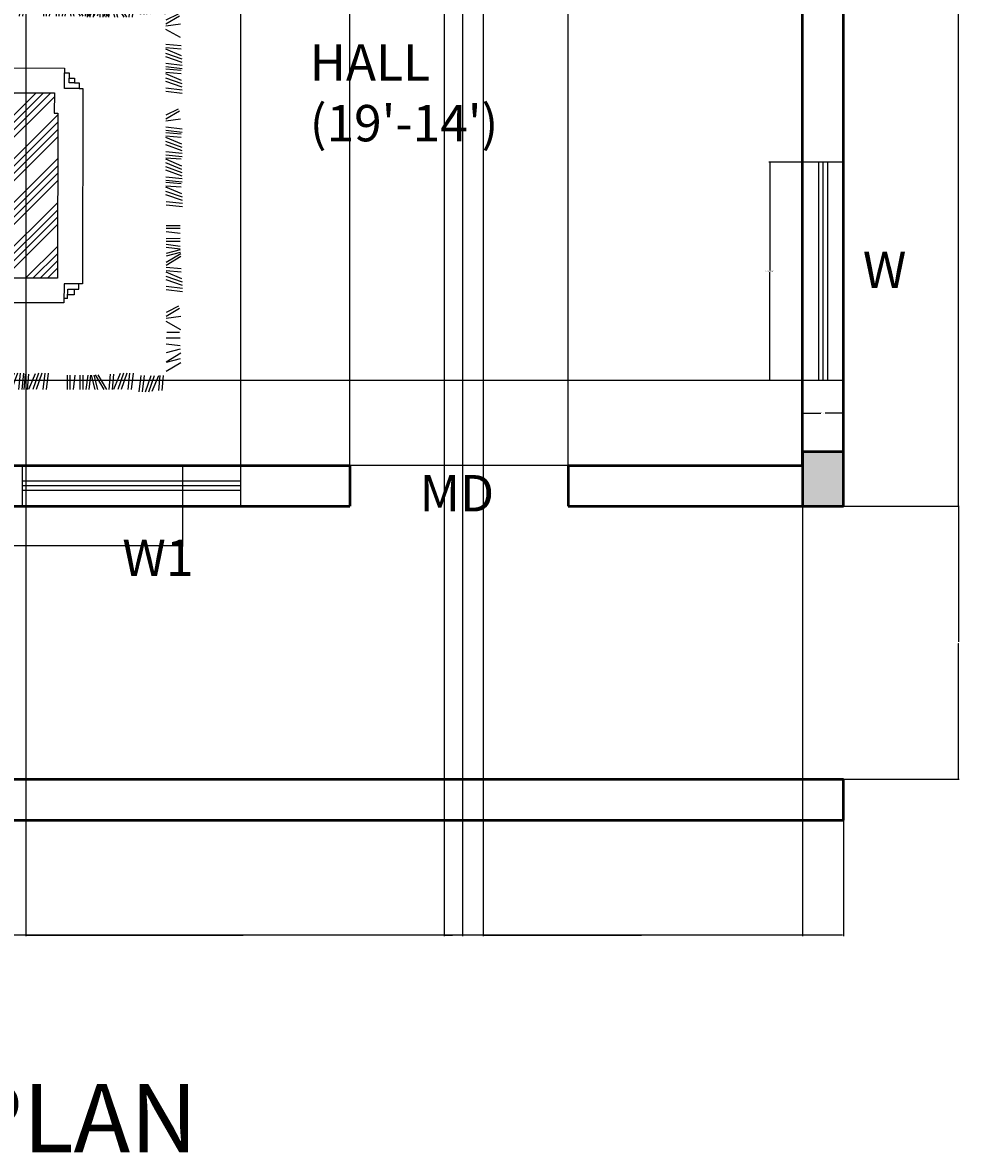
# Model space of a CAD drawing. Units: inches. Extents: x -1517 to -668, y -425 to 52.
# Tile 6 of 13: x -1186 to -980, y -425 to -176. Entities that reach past the tile are written whole.
import ezdxf

# ---------------------------------------------------------------- set-up
doc = ezdxf.new("R2010")
doc.units = ezdxf.units.IN
doc.header["$MEASUREMENT"] = 0
for name, color, linetype, lineweight in [('A-ANNO-DIMS', 2, 'Continuous', 18), ('A-ANNO-TEXT', 7, 'Continuous', 18), ('A-AREA-IDEN', 7, 'Continuous', 25), ('A-COLS-PATT', 252, 'Continuous', 13), ('column', 7, 'Continuous', 50), ('furniture block', 8, 'Continuous', 18), ('walls', 240, 'Continuous', 50), ('windows', 140, 'Continuous', 25)]:
    doc.layers.add(name, color=color, linetype=linetype, lineweight=lineweight)
for name, color, linetype in [('复线', 6, 'Continuous'), ('家具', 4, 'Continuous'), ('辅助线', 1, 'Continuous'), ('门窗', 2, 'Continuous')]:
    doc.layers.add(name, color=color, linetype=linetype)
doc.styles.get("Standard").update_dxf_attribs({"font": 'arial.ttf'})
doc.dimstyles.get("Standard").update_dxf_attribs({"dimtxt": 0.18, "dimasz": 0.18, "dimexe": 0.18, "dimexo": 0.0625, "dimgap": 0.09, "dimtad": 0, "dimtih": 1, "dimtoh": 1, "dimdec": 4, "dimzin": 0, "dimdsep": 46, "dimlunit": 4, "dimtxsty": 'Standard', "dimcen": 0.09, "dimadec": 0, "dimazin": 0, "dimtfac": 1, "dimtdec": 4, "dimtofl": 0, "dimtmove": 0, "dimatfit": 3, "dimfxl": 1, "dimtolj": 1, "dimtzin": 0, "dimarcsym": 0})

# ---------------------------------------------------------------- blocks, each defined once
blk = doc.blocks.new('column')
for p, q in [((0, 9), (0, 0)), ((12, 9), (0, 9)), ((12, 0), (12, 9)), ((0, 0), (12, 0))]:
    blk.add_line(p, q)
blk = doc.blocks.new('window 4ft')
for p, q in [((0, 9), (0, 0)), ((48, 9), (48, 0)), ((0, 5.5), (48, 5.5)), ((0, 4.5), (48, 4.5)), ((0, 3.5), (48, 3.5))]:
    blk.add_line(p, q)
blk = doc.blocks.new('A$C2A9E403C')
at = {"layer": '复线'}
for p, q in [((-0.6124, 1.2901), (-0.6119, 1.5387)), ((-0.6119, 1.5387), (-0.4956, 1.5385)), ((-0.4956, 1.5596), (0.4554, 1.5575)), ((-0.4956, 1.5385), (-0.4956, 1.5596)), ((0.4554, 1.5575), (0.4547, 1.198)), ((-0.5913, 1.2901), (-0.6124, 1.2901)), ((-0.5915, 1.1738), (-0.5913, 1.2901)), ((0.3437, 1.1718), (-0.5915, 1.1738)), ((0.3437, 1.1982), (0.3437, 1.1718)), ((0.4547, 1.198), (0.3437, 1.1982)), ((0.7969, 0.7406), (-0.7994, 0.7387)), ((-0.27, 0.7177), (-0.7787, 0.7173)), ((-0.7787, 0.7173), (-0.7783, 0.1924)), ((-0.2696, 0.1928), (-0.27, 0.7177)), ((0.2616, 0.7183), (-0.2471, 0.718)), ((-0.2471, 0.718), (-0.2468, 0.1931)), ((0.2619, 0.1934), (0.2616, 0.7183)), ((0.7846, 0.7189), (0.2759, 0.7186)), ((0.2759, 0.7186), (0.2762, 0.1937)), ((0.785, 0.194), (0.7846, 0.7189)), ((-1.3039, 0.62), (-1.3039, 0.3666)), ((1.2704, 0.6186), (1.2704, 0.3652)), ((-1.1772, 0.4933), (-1.4306, 0.4933)), ((1.3971, 0.4919), (1.1437, 0.4919)), ((-0.7783, 0.1924), (-0.2696, 0.1928)), ((-0.2468, 0.1931), (0.2619, 0.1934)), ((0.2762, 0.1937), (0.785, 0.194))]:
    blk.add_line(p, q, dxfattribs=at)
for centre in [(-1.2867, 0.4933), (1.2877, 0.4919)]:
    blk.add_circle(centre, 0.0634, dxfattribs=at)
at = {"layer": '家具'}
for p, q in [((0.6497, 2.19), (0.6526, 2.1827)), ((-0.6379, 1.6813), (-0.6378, 1.7025)), ((-0.6378, 1.7025), (0.4874, 1.7)), ((0.4874, 1.7), (0.4872, 1.5943)), ((-0.6961, 1.655), (-0.6696, 1.655)), ((-0.6961, 1.6233), (-0.6961, 1.655)), ((-0.6696, 1.6814), (-0.6379, 1.6813)), ((-0.6696, 1.655), (-0.6696, 1.6814)), ((-0.6694, 1.655), (-0.6694, 1.6235)), ((-0.6378, 1.6814), (-0.6379, 1.597)), ((0.519, 1.6788), (0.4873, 1.6789)), ((0.5189, 1.6154), (0.519, 1.6788)), ((0.519, 1.6524), (0.5507, 1.6523)), ((0.5507, 1.6523), (0.5506, 1.6153)), ((-0.7553, 1.1479), (-0.7543, 1.597)), ((-0.7543, 1.597), (-0.7279, 1.597)), ((-0.6379, 1.597), (-0.7282, 1.5972)), ((-0.7279, 1.597), (-0.7278, 1.6234)), ((-0.7278, 1.6234), (-0.6961, 1.6233)), ((-0.6694, 1.6235), (-0.6966, 1.6235)), ((0.4872, 1.5943), (0.5981, 1.5941)), ((0.5717, 1.6153), (0.5189, 1.6154)), ((0.5717, 1.6153), (0.5717, 1.5941)), ((0.5981, 1.5941), (0.5971, 1.1396)), ((-0.7341, 1.1478), (-0.7553, 1.1479)), ((-0.6393, 1.1482), (-0.7352, 1.1484)), ((-0.7342, 1.1161), (-0.7341, 1.1478)), ((-0.7342, 1.1161), (-0.6972, 1.116)), ((-0.6709, 1.116), (-0.6979, 1.1161)), ((-0.6973, 1.0896), (-0.6972, 1.116)), ((-0.6709, 1.0896), (-0.6709, 1.116)), ((-0.6394, 1.058), (-0.6393, 1.1482)), ((0.4862, 1.1399), (0.4859, 1.0289)), ((0.4862, 1.1399), (0.5971, 1.1396)), ((0.5177, 1.0553), (0.5178, 1.1134)), ((0.5178, 1.1134), (0.5706, 1.1133)), ((0.5442, 1.1133), (0.5441, 1.0816)), ((0.5707, 1.1397), (0.5706, 1.1133)), ((-0.6709, 1.0896), (-0.6973, 1.0896)), ((-0.671, 1.0579), (-0.6709, 1.0896)), ((-0.6393, 1.0578), (-0.671, 1.0579)), ((-0.6393, 1.0314), (-0.6393, 1.0578)), ((0.5177, 1.0553), (0.486, 1.0553)), ((0.5441, 1.0816), (0.5177, 1.0817)), ((0.4859, 1.0289), (-0.6393, 1.0314)), ((-1.549, 0.751), (-1.0422, 0.7516)), ((-1.5485, 0.2441), (-1.549, 0.751)), ((-1.0422, 0.7516), (-1.0416, 0.2447)), ((-0.9818, 0.2137), (-0.9824, 0.7352)), ((-0.7945, 0.7328), (-0.7941, 0.1426)), ((0.7969, 0.7406), (0.7973, 0.1532)), ((0.9782, 0.2083), (0.9775, 0.741)), ((1.0263, 0.7379), (1.5332, 0.7385)), ((1.0269, 0.2311), (1.0263, 0.7379)), ((1.5332, 0.7385), (1.5338, 0.2316)), ((-1.0416, 0.2447), (-1.5485, 0.2441)), ((1.5338, 0.2316), (1.0269, 0.2311)), ((-0.7773, -0.0005), (0.7773, 0.0005))]:
    blk.add_line(p, q, dxfattribs=at)
for centre in [(-1.3039, 0.4933), (1.2704, 0.4919)]:
    blk.add_circle(centre, 0.1267, dxfattribs=at)
for centre, radius, start, end in [((-0.8894, 0.6597), 0.1198, 37.63003, 140.94625), ((0.8885, 0.6609), 0.1198, 41.79306, 142.44625), ((-0.7672, 0.2138), 0.2146, 180.03814, 267.3174), ((0.7771, 0.2016), 0.2011, 270.03814, 1.88757), ((-0.6554, -0.0689), 0.253, 103.34083, 123.25708), ((-0.3975, -0.0687), 0.253, 56.82018, 76.73545), ((-0.1227, -0.0686), 0.253, 59.39874, 122.94271), ((0.1299, -0.0495), 0.2341, 53.21137, 121.92426), ((0.4167, -0.0682), 0.253, 103.34083, 125.41455), ((0.6746, -0.068), 0.253, 60.98187, 76.73545)]:
    blk.add_arc(centre, radius, start, end, dxfattribs=at)
at = {"layer": '辅助线'}
for p, q in [((-1.0661, 2.2523), (-1.0302, 2.1808)), ((-1.0533, 2.2588), (-1.0079, 2.1808)), ((-1.0082, 2.2653), (-0.9957, 2.1808)), ((-0.9309, 2.2654), (-0.9778, 2.1808)), ((-0.8827, 2.2686), (-0.8899, 2.1809)), ((-0.8633, 2.2687), (-0.8705, 2.181)), ((-0.8247, 2.2719), (-0.8633, 2.181)), ((-0.8054, 2.2752), (-0.8391, 2.181)), ((-0.7861, 2.2752), (-0.8197, 2.181)), ((-0.77, 2.2752), (-0.7803, 2.1811)), ((-0.7507, 2.2752), (-0.761, 2.1811)), ((-0.741, 2.2688), (-0.7482, 2.1811)), ((-0.7217, 2.2688), (-0.7289, 2.1811)), ((-0.6831, 2.2721), (-0.7216, 2.1811)), ((-0.6638, 2.2753), (-0.6974, 2.1812)), ((-0.6444, 2.2753), (-0.6781, 2.1812)), ((-0.6284, 2.2754), (-0.6387, 2.1812)), ((-0.609, 2.2754), (-0.6194, 2.1812)), ((-0.5189, 2.253), (-0.483, 2.1814)), ((-0.506, 2.2594), (-0.4607, 2.1814)), ((-0.4609, 2.2659), (-0.4484, 2.1814)), ((-0.4036, 2.2756), (-0.414, 2.1815)), ((-0.3843, 2.2757), (-0.3946, 2.1815)), ((-0.3746, 2.2692), (-0.3818, 2.1815)), ((-0.3553, 2.2693), (-0.3625, 2.1815)), ((-0.3167, 2.2725), (-0.3552, 2.1816)), ((-0.2974, 2.2758), (-0.331, 2.1816)), ((-0.278, 2.2758), (-0.3117, 2.1816)), ((-0.262, 2.2758), (-0.2723, 2.1816)), ((-0.2426, 2.2758), (-0.253, 2.1817)), ((-0.2292, 2.2694), (-0.2364, 2.1817)), ((-0.1906, 2.2727), (-0.2291, 2.1817)), ((-0.1712, 2.2727), (-0.2098, 2.1817)), ((-0.1519, 2.2759), (-0.1856, 2.1817)), ((-0.1326, 2.2759), (-0.1663, 2.1818)), ((-0.1165, 2.276), (-0.1269, 2.1818)), ((-0.0972, 2.276), (-0.1076, 2.1818)), ((-0.0875, 2.2696), (-0.0948, 2.1819)), ((-0.0682, 2.2696), (-0.0754, 2.1819)), ((-0.0296, 2.2728), (-0.0682, 2.1819)), ((-0.0103, 2.2761), (-0.044, 2.1819)), ((0.009, 2.2761), (-0.0246, 2.1819)), ((0.0251, 2.2761), (0.0148, 2.182)), ((0.0444, 2.2761), (0.0341, 2.182)), ((0.1539, 2.2634), (0.154, 2.1821)), ((0.17, 2.2634), (0.1701, 2.1822)), ((0.199, 2.2635), (0.1882, 2.1822)), ((0.2279, 2.2635), (0.228, 2.1822)), ((0.244, 2.2635), (0.2441, 2.1822)), ((0.273, 2.2635), (0.2623, 2.1823)), ((0.2891, 2.2636), (0.2783, 2.1823)), ((0.2923, 2.2636), (0.3127, 2.1823)), ((0.3084, 2.2636), (0.3288, 2.1823)), ((0.3148, 2.2668), (0.3657, 2.1824)), ((0.3309, 2.2668), (0.3818, 2.1824)), ((0.4018, 2.2701), (0.3945, 2.1824)), ((0.4211, 2.2702), (0.4139, 2.1824)), ((0.4597, 2.2734), (0.4211, 2.1825)), ((0.479, 2.2767), (0.4453, 2.1825)), ((0.4983, 2.2767), (0.4647, 2.1825)), ((0.5144, 2.2767), (0.5041, 2.1825)), ((0.5337, 2.2767), (0.5234, 2.1826)), ((0.6175, 2.2543), (0.6497, 2.19)), ((0.6303, 2.2607), (0.6756, 2.1827)), ((0.6754, 2.2672), (0.6879, 2.1828)), ((0.7526, 2.2673), (0.7058, 2.1828)), ((0.7668, 2.187), (0.7667, 2.2602)), ((0.8009, 2.2642), (0.801, 2.1829)), ((0.846, 2.2642), (0.8352, 2.1829)), ((0.8653, 2.2642), (0.8857, 2.183)), ((0.8878, 2.2675), (0.9387, 2.1831)), ((0.92, 2.2643), (0.9405, 2.1831)), ((0.9426, 2.2675), (0.9934, 2.1831)), ((-1.1526, 2.1822), (-1.0649, 2.175)), ((1.1031, 2.1597), (1.0154, 2.1669)), ((-1.1494, 2.1339), (-1.0648, 2.0871)), ((1.1031, 2.1404), (1.0154, 2.1476)), ((1.1064, 2.1018), (1.0154, 2.1404)), ((1.1096, 2.0825), (1.0155, 2.1161)), ((1.1097, 2.0632), (1.0155, 2.0968)), ((-1.1493, 2.0567), (-1.0648, 2.0692)), ((-1.1428, 2.0116), (-1.0648, 2.0569)), ((-1.1205, 2.0067), (-1.0648, 2.0347)), ((1.1097, 2.0471), (1.0155, 2.0574)), ((1.1097, 2.0278), (1.0156, 2.0381)), ((-1.1354, 1.9942), (-1.0477, 1.987)), ((-1.1354, 1.9749), (-1.0477, 1.9677)), ((-1.1321, 1.9041), (-1.0476, 1.9549)), ((1.0017, 1.9919), (1.0958, 1.9816)), ((1.0017, 1.9726), (1.0958, 1.9623)), ((1.0017, 1.9565), (1.0959, 1.9229)), ((-1.132, 1.888), (-1.0476, 1.9389)), ((-1.1288, 1.8816), (-1.0476, 1.902)), ((1.0017, 1.9372), (1.0959, 1.9036)), ((1.005, 1.9179), (1.0959, 1.8793)), ((-1.1487, 1.855), (-1.0545, 1.8446)), ((-1.1486, 1.8356), (-1.0545, 1.8253)), ((-1.1288, 1.8655), (-1.0476, 1.8859)), ((-1.1288, 1.8623), (-1.0475, 1.8515)), ((-1.1288, 1.8462), (-1.0475, 1.8354)), ((1.0082, 1.8793), (1.0959, 1.8721)), ((1.0083, 1.86), (1.096, 1.8528)), ((1.0116, 1.7892), (1.096, 1.84)), ((1.0116, 1.7731), (1.096, 1.8239)), ((-1.1486, 1.8196), (-1.0544, 1.7859)), ((-1.1486, 1.8002), (-1.0544, 1.7666)), ((-1.1454, 1.7809), (-1.0544, 1.7424)), ((-1.1287, 1.8172), (-1.0475, 1.8173)), ((-1.1287, 1.8011), (-1.0475, 1.8012)), ((-1.1287, 1.7721), (-1.0474, 1.7614)), ((1.0148, 1.7666), (1.096, 1.787)), ((1.0148, 1.7505), (1.0961, 1.771)), ((-1.1421, 1.7423), (-1.0544, 1.7351)), ((-1.1421, 1.723), (-1.0544, 1.7158)), ((-1.1388, 1.6522), (-1.0544, 1.703)), ((-1.1287, 1.7432), (-1.0474, 1.7433)), ((-1.1286, 1.7271), (-1.0474, 1.7272)), ((1.0148, 1.7473), (1.0961, 1.7366)), ((1.0148, 1.7312), (1.0961, 1.7205)), ((1.0149, 1.7022), (1.0961, 1.7023)), ((-1.1388, 1.6361), (-1.0543, 1.6869)), ((-1.1355, 1.6296), (-1.0543, 1.6501)), ((-1.1355, 1.6135), (-1.0543, 1.634)), ((1.0149, 1.6861), (1.0962, 1.6862)), ((1.0149, 1.6572), (1.0962, 1.6464)), ((1.015, 1.6282), (1.0962, 1.6283)), ((-1.1355, 1.6103), (-1.0542, 1.5996)), ((-1.1355, 1.5942), (-1.0542, 1.5835)), ((-1.1355, 1.5653), (-1.0542, 1.5654)), ((1.015, 1.6121), (1.0962, 1.6122)), ((-1.1354, 1.5492), (-1.0542, 1.5493)), ((-1.1354, 1.5202), (-1.0541, 1.5094)), ((-0.2678, 1.1731), (-0.6119, 1.5187)), ((-0.2258, 1.173), (-0.5898, 1.5387)), ((-0.0998, 1.1727), (-0.4849, 1.5596)), ((-0.0578, 1.1727), (-0.4429, 1.5595)), ((-0.0158, 1.1726), (-0.4009, 1.5594)), ((0.0262, 1.1725), (-0.3589, 1.5593)), ((0.1522, 1.1722), (-0.2329, 1.559)), ((0.1942, 1.1721), (-0.1909, 1.5589)), ((0.2362, 1.172), (-0.1489, 1.5588)), ((0.2782, 1.1719), (-0.1069, 1.5587)), ((0.3779, 1.1981), (0.0191, 1.5585)), ((0.4199, 1.198), (0.0611, 1.5584)), ((0.4547, 1.2052), (0.1031, 1.5583)), ((0.4548, 1.2472), (0.1451, 1.5582)), ((0.455, 1.3732), (0.2711, 1.5579)), ((0.4551, 1.4152), (0.3131, 1.5578)), ((0.4552, 1.4572), (0.3551, 1.5577)), ((0.4553, 1.4992), (0.3971, 1.5576)), ((1.0022, 1.5026), (1.0964, 1.4923)), ((-1.1354, 1.4912), (-1.0541, 1.4913)), ((-1.1354, 1.4751), (-1.0541, 1.4752)), ((-0.3518, 1.1733), (-0.6121, 1.4347)), ((-0.3098, 1.1732), (-0.612, 1.4767)), ((1.0023, 1.4833), (1.0964, 1.473)), ((1.0023, 1.4672), (1.0965, 1.4336)), ((1.0023, 1.4479), (1.0965, 1.4143)), ((1.0055, 1.4286), (1.0965, 1.39)), ((1.0088, 1.39), (1.0965, 1.3828)), ((1.0088, 1.3707), (1.0965, 1.3635)), ((-1.1481, 1.3657), (-1.0539, 1.3553)), ((-1.1481, 1.3463), (-1.0539, 1.336)), ((-1.1481, 1.3303), (-1.0539, 1.2966)), ((-1.148, 1.3109), (-1.0539, 1.2773)), ((-0.5938, 1.2901), (-0.6124, 1.3087)), ((1.0024, 1.361), (1.0966, 1.3506)), ((1.0024, 1.3417), (1.0966, 1.3313)), ((1.0024, 1.3256), (1.0966, 1.2919)), ((1.0025, 1.3063), (1.0966, 1.2726)), ((-1.1448, 1.2916), (-1.0538, 1.2531)), ((-1.1415, 1.253), (-1.0538, 1.2458)), ((-0.5198, 1.1737), (-0.5914, 1.2456)), ((-0.4778, 1.1736), (-0.5913, 1.2876)), ((1.0057, 1.287), (1.0967, 1.2484)), ((1.0057, 1.2677), (1.0967, 1.2291)), ((-1.1479, 1.224), (-1.0538, 1.2137)), ((-1.1479, 1.2047), (-1.0538, 1.1944)), ((-1.1479, 1.1886), (-1.0537, 1.155)), ((-1.1415, 1.2337), (-1.0538, 1.2265)), ((-0.5618, 1.1738), (-0.5915, 1.2036)), ((1.0026, 1.2156), (1.0967, 1.2052)), ((1.0026, 1.1963), (1.0967, 1.1859)), ((1.0026, 1.1802), (1.0968, 1.1465)), ((1.009, 1.229), (1.0967, 1.2218)), ((-1.1479, 1.1693), (-1.0537, 1.1356)), ((-1.1446, 1.15), (-1.0537, 1.1114)), ((-1.1446, 1.1307), (-1.0536, 1.0921)), ((1.0026, 1.1608), (1.0968, 1.1272)), ((1.0059, 1.1415), (1.0968, 1.103)), ((-1.1478, 1.0786), (-1.0536, 1.0682)), ((-1.1477, 1.0593), (-1.0536, 1.0489)), ((-1.1477, 1.0432), (-1.0535, 1.0095)), ((-1.1413, 1.0921), (-1.0536, 1.0848)), ((1.0027, 1.0739), (1.0969, 1.0636)), ((1.0028, 1.0546), (1.0969, 1.0443)), ((1.0091, 1.1029), (1.0968, 1.0957)), ((1.0092, 1.0836), (1.0969, 1.0764)), ((-1.1477, 1.0239), (-1.0535, 0.9902)), ((-1.1445, 1.0046), (-1.0535, 0.966)), ((1.0125, 0.9973), (1.0969, 1.0098)), ((1.019, 0.9522), (1.097, 0.9975)), ((-1.1476, 0.937), (-1.0535, 0.9266)), ((-1.1476, 0.9176), (-1.0534, 0.9073)), ((-1.1412, 0.9659), (-1.0535, 0.9587)), ((-1.1412, 0.9466), (-1.0535, 0.9394)), ((1.0182, 0.9266), (1.1091, 0.8881)), ((1.0254, 0.9393), (1.097, 0.9752)), ((-1.1379, 0.8603), (-1.0534, 0.8728)), ((-1.1314, 0.8152), (-1.0534, 0.8605)), ((1.015, 0.8745), (1.1091, 0.8642)), ((1.015, 0.8552), (1.1092, 0.8449)), ((1.0214, 0.888), (1.1091, 0.8808)), ((-1.1353, 0.8078), (-1.062, 0.8079)), ((-1.132, 0.8163), (-1.0631, 0.7916)), ((-1.1249, 0.8024), (-1.0533, 0.8383)), ((-1.0607, 0.8176), (-1.0606, 0.7516)), ((1.015, 0.8391), (1.1092, 0.8055)), ((1.0151, 0.7984), (1.0863, 0.8153)), ((1.0173, 0.7141), (1.0171, 0.8166)), ((1.0174, 0.7888), (1.0906, 0.7889)), ((-1.5237, 0.7257), (-1.0675, 0.7262)), ((-1.5231, 0.2695), (-1.5237, 0.7257)), ((-1.1351, 0.7732), (-1.0621, 0.7791)), ((-1.135, 0.7635), (-1.0628, 0.7759)), ((-1.0675, 0.7262), (-1.067, 0.27)), ((1.0164, 0.7803), (1.0847, 0.754)), ((1.0189, 0.7534), (1.0705, 0.738)), ((-1.0421, 0.7117), (-0.9824, 0.7118)), ((-1.0339, 0.6392), (-1.0219, 0.7114)), ((-1.0207, 0.6402), (-1.0046, 0.7117)), ((-0.9891, 0.6447), (-1.0003, 0.7117)), ((-0.7461, 0.6679), (-0.7458, 0.227)), ((-0.316, 0.6798), (-0.7345, 0.6795)), ((-0.3041, 0.2273), (-0.3044, 0.6682)), ((-0.2146, 0.6685), (-0.2143, 0.2277)), ((0.2155, 0.6804), (-0.203, 0.6801)), ((0.2275, 0.228), (0.2272, 0.6688)), ((0.3111, 0.6701), (0.3114, 0.2287)), ((0.7428, 0.682), (0.3227, 0.6817)), ((0.7547, 0.229), (0.7544, 0.6704)), ((0.9776, 0.714), (1.0173, 0.7141)), ((0.988, 0.6409), (0.9879, 0.7142)), ((1.0156, 0.6423), (1.004, 0.7146)), ((1.0149, 0.641), (1.0148, 0.7142)), ((1.0517, 0.7126), (1.5079, 0.7131)), ((1.0522, 0.2564), (1.0517, 0.7126)), ((1.5079, 0.7131), (1.5084, 0.257)), ((-1.067, 0.27), (-1.5231, 0.2695)), ((-0.7458, 0.227), (-0.3041, 0.2273)), ((-0.2143, 0.2277), (0.2275, 0.228)), ((0.3114, 0.2287), (0.7547, 0.229)), ((1.5084, 0.257), (1.0522, 0.2564))]:
    blk.add_line(p, q, dxfattribs=at)
for centre, start, end in [((-0.7345, 0.6679), 90.03814, 180.03814), ((-0.316, 0.6682), 0.03814, 90.03814), ((-0.203, 0.6685), 90.03814, 180.03814), ((0.2156, 0.6688), 0.03814, 90.03814), ((0.3228, 0.6701), 90.03814, 180.03814), ((0.7428, 0.6703), 0.03814, 90.03814)]:
    blk.add_arc(centre, 0.0116, start, end, dxfattribs=at)
at = {"layer": '门窗'}
for centre, radius, start, end in [((-0.5259, -0.9226), 1.1183, 84.44463, 95.63165), ((0.5462, -0.9219), 1.1183, 84.44463, 95.63165), ((-0.5778, -0.396), 0.5891, 95.63165, 103.34083), ((-0.4747, -0.3959), 0.5891, 76.73545, 84.44463), ((0.4943, -0.3953), 0.5891, 95.63165, 103.34083), ((0.5974, -0.3952), 0.5891, 76.73545, 84.44463)]:
    blk.add_arc(centre, radius, start, end, dxfattribs=at)
blk = doc.blocks.new('*D24')
at = {"layer": 'A-ANNO-DIMS', "color": 0, "lineweight": -2, "transparency": 16777216}
for p, q in [((-1014.57, -206.68), (-1021.88, -206.68)), ((-1021.7, -206.86), (-1021.7, -230.5)), ((-1021.7, -254.5), (-1021.7, -230.87)), ((-1014.57, -254.68), (-1021.88, -254.68))]:
    blk.add_line(p, q, dxfattribs=at)
at = {"layer": 'A-ANNO-DIMS', "color": 0, "transparency": 16777216}
for points in [[(-1021.73, -206.86), (-1021.67, -206.86), (-1021.7, -206.68)], [(-1021.73, -254.5), (-1021.67, -254.5), (-1021.7, -254.68)]]:
    blk.add_solid(points, dxfattribs=at)
at = {"layer": 'Defpoints', "color": 0, "transparency": 16777216}
for p in [(-1014.5, -206.68), (-1021.7, -254.68), (-1014.5, -254.68)]:
    blk.add_point(p, dxfattribs=at)
at = {"layer": 'A-ANNO-DIMS', "color": 0, "transparency": 16777216, "insert": (-1021.7, -230.68), "char_height": 0.18, "attachment_point": 5}
blk.add_mtext('\\A1;WINDOW 48 TYP.', dxfattribs=at)
blk = doc.blocks.new('*D25')
at = {"layer": 'A-ANNO-DIMS', "color": 0, "lineweight": -2, "transparency": 16777216}
for p, q in [((-1014.5, -254.75), (-1014.5, -262.06)), ((-1005.5, -254.75), (-1005.5, -262.06)), ((-1014.32, -261.88), (-1010.46, -261.88)), ((-1005.68, -261.88), (-1009.55, -261.88))]:
    blk.add_line(p, q, dxfattribs=at)
at = {"layer": 'A-ANNO-DIMS', "color": 0, "transparency": 16777216}
for points in [[(-1014.32, -261.85), (-1014.32, -261.91), (-1014.5, -261.88)], [(-1005.68, -261.85), (-1005.68, -261.91), (-1005.5, -261.88)]]:
    blk.add_solid(points, dxfattribs=at)
at = {"layer": 'Defpoints', "color": 0, "transparency": 16777216}
for p in [(-1014.5, -254.68), (-1005.5, -254.68), (-1005.5, -261.88)]:
    blk.add_point(p, dxfattribs=at)
at = {"layer": 'A-ANNO-DIMS', "color": 0, "transparency": 16777216, "insert": (-1010, -261.88), "char_height": 0.18, "attachment_point": 5}
blk.add_mtext('\\A1;9 TYP.', dxfattribs=at)
blk = doc.blocks.new('*D43')
at = {"layer": 'A-ANNO-DIMS', "color": 0, "lineweight": -2, "transparency": 16777216}
for p, q in [((-1237.78, -273.43), (-1237.78, -291.2)), ((-1150.87, -273.43), (-1150.87, -291.2)), ((-1237.6, -291.02), (-1194.54, -291.02)), ((-1151.05, -291.02), (-1194.1, -291.02))]:
    blk.add_line(p, q, dxfattribs=at)
at = {"layer": 'A-ANNO-DIMS', "color": 0, "transparency": 16777216}
for points in [[(-1237.6, -290.99), (-1237.6, -291.05), (-1237.78, -291.02)], [(-1151.05, -290.99), (-1151.05, -291.05), (-1150.87, -291.02)]]:
    blk.add_solid(points, dxfattribs=at)
at = {"layer": 'Defpoints', "color": 0, "transparency": 16777216}
for p in [(-1237.78, -273.37), (-1150.87, -273.37), (-1150.87, -291.02)]:
    blk.add_point(p, dxfattribs=at)
at = {"layer": 'A-ANNO-DIMS', "color": 0, "transparency": 16777216, "insert": (-1194.32, -291.02), "char_height": 0.18, "attachment_point": 5}
blk.add_mtext('\\A1;87', dxfattribs=at)
blk = doc.blocks.new('*D44')
at = {"layer": 'A-ANNO-DIMS', "color": 0, "lineweight": -2, "transparency": 16777216}
for p, q in [((-1491.5, -351.43), (-1491.5, -376.85)), ((-1005.5, -351.43), (-1005.5, -376.85)), ((-1491.32, -376.67), (-1248.8, -376.67)), ((-1005.68, -376.67), (-1248.21, -376.67))]:
    blk.add_line(p, q, dxfattribs=at)
at = {"layer": 'A-ANNO-DIMS', "color": 0, "transparency": 16777216}
for points in [[(-1491.32, -376.64), (-1491.32, -376.7), (-1491.5, -376.67)], [(-1005.68, -376.64), (-1005.68, -376.7), (-1005.5, -376.67)]]:
    blk.add_solid(points, dxfattribs=at)
at = {"layer": 'Defpoints', "color": 0, "transparency": 16777216}
for p in [(-1491.5, -351.37), (-1005.5, -351.37), (-1005.5, -376.67)]:
    blk.add_point(p, dxfattribs=at)
at = {"layer": 'A-ANNO-DIMS', "color": 0, "transparency": 16777216, "insert": (-1248.5, -376.67), "char_height": 0.18, "attachment_point": 5}
blk.add_mtext('\\A1;486', dxfattribs=at)
blk = doc.blocks.new('*D46')
at = {"layer": 'A-ANNO-DIMS', "color": 0, "lineweight": -2, "transparency": 16777216}
for p, q in [((-1005.44, 26.63), (-980.02, 26.63)), ((-980.2, 26.45), (-980.2, -127.69)), ((-980.2, -282.19), (-980.2, -128.05)), ((-1005.44, -282.37), (-980.02, -282.37))]:
    blk.add_line(p, q, dxfattribs=at)
at = {"layer": 'A-ANNO-DIMS', "color": 0, "transparency": 16777216}
for points in [[(-980.23, 26.45), (-980.17, 26.45), (-980.2, 26.63)], [(-980.23, -282.19), (-980.17, -282.19), (-980.2, -282.37)]]:
    blk.add_solid(points, dxfattribs=at)
at = {"layer": 'Defpoints', "color": 0, "transparency": 16777216}
for p in [(-1005.5, 26.63), (-1005.5, -282.37), (-980.2, -282.37)]:
    blk.add_point(p, dxfattribs=at)
at = {"layer": 'A-ANNO-DIMS', "color": 0, "transparency": 16777216, "insert": (-980.2, -127.87), "char_height": 0.18, "attachment_point": 5}
blk.add_mtext('\\A1;309', dxfattribs=at)
blk = doc.blocks.new('*D49')
at = {"layer": 'A-ANNO-DIMS', "color": 0, "lineweight": -2, "transparency": 16777216}
for p, q in [((-1185.3, -102.43), (-1185.3, -376.85)), ((-1089.3, -102.43), (-1089.3, -376.85)), ((-1185.12, -376.67), (-1137.52, -376.67)), ((-1089.48, -376.67), (-1137.08, -376.67))]:
    blk.add_line(p, q, dxfattribs=at)
at = {"layer": 'A-ANNO-DIMS', "color": 0, "transparency": 16777216}
for points in [[(-1185.12, -376.64), (-1185.12, -376.7), (-1185.3, -376.67)], [(-1089.48, -376.64), (-1089.48, -376.7), (-1089.3, -376.67)]]:
    blk.add_solid(points, dxfattribs=at)
at = {"layer": 'Defpoints', "color": 0, "transparency": 16777216}
for p in [(-1185.3, -102.37), (-1089.3, -102.37), (-1089.3, -376.67)]:
    blk.add_point(p, dxfattribs=at)
at = {"layer": 'A-ANNO-DIMS', "color": 0, "transparency": 16777216, "insert": (-1137.3, -376.67), "char_height": 0.18, "attachment_point": 5}
blk.add_mtext('\\A1;96', dxfattribs=at)
blk = doc.blocks.new('*D50')
at = {"layer": 'A-ANNO-DIMS', "color": 0, "lineweight": -2, "transparency": 16777216}
for p, q in [((-1084.7, -102.43), (-1084.7, -376.85)), ((-1014.5, -102.43), (-1014.5, -376.85)), ((-1084.52, -376.67), (-1049.93, -376.67)), ((-1014.68, -376.67), (-1049.28, -376.67))]:
    blk.add_line(p, q, dxfattribs=at)
at = {"layer": 'A-ANNO-DIMS', "color": 0, "transparency": 16777216}
for points in [[(-1084.52, -376.64), (-1084.52, -376.7), (-1084.7, -376.67)], [(-1014.68, -376.64), (-1014.68, -376.7), (-1014.5, -376.67)]]:
    blk.add_solid(points, dxfattribs=at)
at = {"layer": 'Defpoints', "color": 0, "transparency": 16777216}
for p in [(-1084.7, -102.37), (-1014.5, -102.37), (-1014.5, -376.67)]:
    blk.add_point(p, dxfattribs=at)
at = {"layer": 'A-ANNO-DIMS', "color": 0, "transparency": 16777216, "insert": (-1049.6, -376.67), "char_height": 0.18, "attachment_point": 5}
blk.add_mtext('\\A1;70.2', dxfattribs=at)
blk = doc.blocks.new('*D57')
at = {"layer": 'A-ANNO-DIMS', "color": 0, "lineweight": -2, "transparency": 16777216}
for p, q in [((-1114.02, -282.31), (-1114.02, 52.11)), ((-1113.84, 51.93), (-1090.24, 51.93)), ((-1066.2, 51.93), (-1089.8, 51.93)), ((-1066.02, -282.31), (-1066.02, 52.11))]:
    blk.add_line(p, q, dxfattribs=at)
at = {"layer": 'A-ANNO-DIMS', "color": 0, "transparency": 16777216}
for points in [[(-1113.84, 51.96), (-1113.84, 51.9), (-1114.02, 51.93)], [(-1066.2, 51.96), (-1066.2, 51.9), (-1066.02, 51.93)]]:
    blk.add_solid(points, dxfattribs=at)
at = {"layer": 'Defpoints', "color": 0, "transparency": 16777216}
for p in [(-1066.02, 51.93), (-1114.02, -282.37), (-1066.02, -282.37)]:
    blk.add_point(p, dxfattribs=at)
at = {"layer": 'A-ANNO-DIMS', "color": 0, "transparency": 16777216, "insert": (-1090.02, 51.93), "char_height": 0.18, "attachment_point": 5}
blk.add_mtext('\\A1;48', dxfattribs=at)
blk = doc.blocks.new('*D58')
at = {"layer": 'A-ANNO-DIMS', "color": 0, "lineweight": -2, "transparency": 16777216}
for p, q in [((-1066.02, -282.31), (-1066.02, 52.11)), ((-1065.84, 51.93), (-1036.14, 51.93)), ((-1005.68, 51.93), (-1035.38, 51.93)), ((-1005.5, -282.31), (-1005.5, 52.11))]:
    blk.add_line(p, q, dxfattribs=at)
at = {"layer": 'A-ANNO-DIMS', "color": 0, "transparency": 16777216}
for points in [[(-1065.84, 51.96), (-1065.84, 51.9), (-1066.02, 51.93)], [(-1005.68, 51.96), (-1005.68, 51.9), (-1005.5, 51.93)]]:
    blk.add_solid(points, dxfattribs=at)
at = {"layer": 'Defpoints', "color": 0, "transparency": 16777216}
for p in [(-1005.5, 51.93), (-1066.02, -282.37), (-1005.5, -282.37)]:
    blk.add_point(p, dxfattribs=at)
at = {"layer": 'A-ANNO-DIMS', "color": 0, "transparency": 16777216, "insert": (-1035.76, 51.93), "char_height": 0.18, "attachment_point": 5}
blk.add_mtext('\\A1;60.51', dxfattribs=at)
blk = doc.blocks.new('*D65')
at = {"layer": 'A-ANNO-DIMS', "color": 0, "lineweight": -2, "transparency": 16777216}
for p, q in [((-1138.02, -282.31), (-1138.02, 52.11)), ((-1137.84, 51.93), (-1126.24, 51.93)), ((-1114.2, 51.93), (-1125.8, 51.93)), ((-1114.02, -282.31), (-1114.02, 52.11))]:
    blk.add_line(p, q, dxfattribs=at)
at = {"layer": 'A-ANNO-DIMS', "color": 0, "transparency": 16777216}
for points in [[(-1137.84, 51.96), (-1137.84, 51.9), (-1138.02, 51.93)], [(-1114.2, 51.96), (-1114.2, 51.9), (-1114.02, 51.93)]]:
    blk.add_solid(points, dxfattribs=at)
at = {"layer": 'Defpoints', "color": 0, "transparency": 16777216}
for p in [(-1114.02, 51.93), (-1138.02, -282.37), (-1114.02, -282.37)]:
    blk.add_point(p, dxfattribs=at)
at = {"layer": 'A-ANNO-DIMS', "color": 0, "transparency": 16777216, "insert": (-1126.02, 51.93), "char_height": 0.18, "attachment_point": 5}
blk.add_mtext('\\A1;24', dxfattribs=at)
blk = doc.blocks.new('*D66')
at = {"layer": 'A-ANNO-DIMS', "color": 0, "lineweight": -2, "transparency": 16777216}
for p, q in [((-1014.57, -254.68), (-1516.98, -254.68)), ((-1516.8, -254.86), (-1516.8, -263.85)), ((-1516.8, -273.19), (-1516.8, -264.21)), ((-1014.57, -273.37), (-1516.98, -273.37))]:
    blk.add_line(p, q, dxfattribs=at)
at = {"layer": 'A-ANNO-DIMS', "color": 0, "transparency": 16777216}
for points in [[(-1516.83, -254.86), (-1516.77, -254.86), (-1516.8, -254.68)], [(-1516.83, -273.19), (-1516.77, -273.19), (-1516.8, -273.37)]]:
    blk.add_solid(points, dxfattribs=at)
at = {"layer": 'Defpoints', "color": 0, "transparency": 16777216}
for p in [(-1014.5, -254.68), (-1516.8, -273.37), (-1014.5, -273.37)]:
    blk.add_point(p, dxfattribs=at)
at = {"layer": 'A-ANNO-DIMS', "color": 0, "transparency": 16777216, "insert": (-1516.8, -264.03), "char_height": 0.18, "attachment_point": 5}
blk.add_mtext('\\A1;18.686', dxfattribs=at)
blk = doc.blocks.new('*D70')
at = {"layer": 'A-ANNO-DIMS', "color": 0, "lineweight": -2, "transparency": 16777216}
for p, q in [((-1089.3, -102.43), (-1089.3, -376.85)), ((-1093.3, -107.03), (-1093.3, -376.85)), ((-1093.12, -376.67), (-1091.46, -376.67)), ((-1089.48, -376.67), (-1091.15, -376.67))]:
    blk.add_line(p, q, dxfattribs=at)
at = {"layer": 'A-ANNO-DIMS', "color": 0, "transparency": 16777216}
for points in [[(-1093.12, -376.64), (-1093.12, -376.7), (-1093.3, -376.67)], [(-1089.48, -376.64), (-1089.48, -376.7), (-1089.3, -376.67)]]:
    blk.add_solid(points, dxfattribs=at)
at = {"layer": 'Defpoints', "color": 0, "transparency": 16777216}
for p in [(-1089.3, -102.37), (-1093.3, -106.97), (-1089.3, -376.67)]:
    blk.add_point(p, dxfattribs=at)
at = {"layer": 'A-ANNO-DIMS', "color": 0, "transparency": 16777216, "insert": (-1091.3, -376.67), "char_height": 0.18, "attachment_point": 5}
blk.add_mtext('\\A1;4', dxfattribs=at)
blk = doc.blocks.new('*D81')
at = {"layer": 'A-ANNO-DIMS', "color": 0, "lineweight": -2, "transparency": 16777216}
for p, q in [((-1005.44, -282.37), (-980.02, -282.37)), ((-980.2, -282.55), (-980.2, -312.19)), ((-980.2, -342.19), (-980.2, -312.55)), ((-1005.44, -342.37), (-980.02, -342.37))]:
    blk.add_line(p, q, dxfattribs=at)
at = {"layer": 'A-ANNO-DIMS', "color": 0, "transparency": 16777216}
for points in [[(-980.23, -282.55), (-980.17, -282.55), (-980.2, -282.37)], [(-980.23, -342.19), (-980.17, -342.19), (-980.2, -342.37)]]:
    blk.add_solid(points, dxfattribs=at)
at = {"layer": 'Defpoints', "color": 0, "transparency": 16777216}
for p in [(-1005.5, -282.37), (-1005.5, -342.37), (-980.2, -342.37)]:
    blk.add_point(p, dxfattribs=at)
at = {"layer": 'A-ANNO-DIMS', "color": 0, "transparency": 16777216, "insert": (-980.2, -312.37), "char_height": 0.18, "attachment_point": 5}
blk.add_mtext('\\A1;60', dxfattribs=at)

msp = doc.modelspace()

# ---------------------------------------------------------------- hatches: boundary and pattern name
at = {"layer": 'A-COLS-PATT'}
h = msp.add_hatch(dxfattribs=at)
h.set_pattern_fill('AR-CONC', color=256, scale=0.69)
h.set_pattern_definition([(50, (0, 0), (4.949095, -0.43299), [0.5175, -5.6925]), (355, (0, 0), (-0.957384, 5.190126), [0.414, -4.554]), (100.45144, (0.4124, -0.036), (3.991711, 4.757136), [0.439807, -4.83788]), (46.1842, (0, 1.38), (7.363965, -1.142083), [0.77625, -8.53875]), (96.63564, (0.614, 1.285), (6.449167, 6.72142), [0.65971, -7.256825]), (351.18416, (0, 1.38), (6.449167, 6.72142), [0.621, -6.831]), (21, (0.69, 1.035), (4.118659, -2.77807), [0.5175, -5.6925]), (326, (0.69, 1.035), (1.678876, 5.003535), [0.414, -4.554]), (71.45144, (1.033, 0.8035), (5.797534, 2.225465), [0.439807, -4.83788]), (37.5, (0, 0), (0.083903, 2.2969676), [0, -4.4988, 0, -4.623, 0, -4.57125]), (7.5, (0, 0), (1.81518, 2.721441), [0, -2.6358, 0, -4.3953, 0, -1.74225]), (327.5, (-1.5387, 0), (3.6833748, -0.1556286), [0, -1.725, 0, -5.382, 0, -7.1415]), (317.5, (-2.2287, 0), (4.0239846, 0.6907244), [0, -2.2425, 0, -3.5742, 0, -5.0715])])
h.paths.add_polyline_path([(-1491.5037, 26.63), (-1491.5037, 17.63), (-1479.5037, 17.63), (-1479.5037, 26.63)])
h.paths.add_polyline_path([(-1278.5037, 17.63), (-1278.5037, 26.63), (-1290.5037, 26.63), (-1290.5037, 17.63)])
h.paths.add_polyline_path([(-1177.9037, 26.63), (-1189.9037, 26.63), (-1189.9037, 17.63), (-1177.9037, 17.63)])
h.paths.add_polyline_path([(-1017.5037, 26.63), (-1017.5037, 17.63), (-1005.5037, 17.63), (-1005.5037, 26.63)])
h.paths.add_polyline_path([(-1005.5037, -270.37), (-1014.5037, -270.37), (-1014.5037, -282.37), (-1005.5037, -282.37)])
h.paths.add_polyline_path([(-1247.1037, -282.37), (-1235.1037, -282.37), (-1235.1037, -273.37), (-1247.1037, -273.37)])
h.paths.add_polyline_path([(-1367.1037, -273.37), (-1367.1037, -282.37), (-1355.1037, -282.37), (-1355.1037, -273.37)])
h.paths.add_polyline_path([(-1491.5037, -282.37), (-1479.5037, -282.37), (-1479.5037, -273.37), (-1491.5037, -273.37)])
h.paths.add_polyline_path([(-1482.5037, -145.97), (-1491.5037, -145.97), (-1491.5037, -157.97), (-1482.5037, -157.97)])
h.paths.add_polyline_path([(-1491.5037, -94.97), (-1491.5037, -106.97), (-1482.5037, -106.97), (-1482.5037, -94.97)])

# ---------------------------------------------------------------- linework, layer by layer
at = {"layer": 'walls'}
for p, q in [((-1005.5037, -282.37), (-1005.5037, 26.63)), ((-1014.5037, -273.37), (-1014.5037, -106.97)), ((-1242.5037, -273.37), (-1114.0183, -273.37)), ((-1114.0183, -273.37), (-1114.0183, -282.37)), ((-1066.0183, -273.37), (-1014.5037, -273.37)), ((-1066.0183, -273.37), (-1066.0183, -282.37)), ((-1482.5037, -282.37), (-1114.0183, -282.37)), ((-1066.0183, -282.37), (-1014.5037, -282.37)), ((-1482.5037, -342.37), (-1014.5037, -342.37)), ((-1014.5037, -342.37), (-1005.5037, -342.37)), ((-1005.5037, -351.37), (-1005.5037, -342.37)), ((-1491.5037, -351.37), (-1005.5037, -351.37))]:
    msp.add_line(p, q, dxfattribs=at)

# ---------------------------------------------------------------- block references
at = {"layer": 'column', "rotation": 270}
msp.add_blockref('column', (-1014.5037, -270.37), dxfattribs=at)
at = {"layer": 'furniture block', "xscale": 38.16622643712981, "yscale": 38.16622643712981, "zscale": 38.16622643712981, "rotation": 270}
msp.add_blockref('A$C2A9E403C', (-1237.7606, -214.8323), dxfattribs=at)
at = {"layer": 'windows'}
for p, rotation in [((-1014.5037, -206.6839), 269.9999999999998), ((-1138.0183, -273.37), 179.9999999999998)]:
    msp.add_blockref('window 4ft', p, dxfattribs=dict(at, rotation=rotation))

# ---------------------------------------------------------------- texts
at = {"layer": 'A-ANNO-TEXT', "attachment_point": 1}
for s, width, insert, char_height in [('{\\fArial|b1|i0|c0|p34;W}', 23.131632, (-1001.236, -226.3617), 8), ('{\\fArial|b1|i0|c0|p34;MD}', 23.131632, (-1098.6962, -275.496), 8), ('{\\fArial|b1|i0|c0|p34;W1 }', 23.131632, (-1164.089, -289.6665), 8), ('{\\fArial|b1|i0|c0|p34;GROUND FLOOR PLAN}', 581.299229, (-1359.7191, -409.3504), 15)]:
    msp.add_mtext_dynamic_manual_height_columns(s, width=width, gutter_width=1, heights=[0], dxfattribs=dict(at, insert=insert, char_height=char_height))
at = {"layer": 'A-AREA-IDEN', "insert": (-1122.8621, -180.8024), "char_height": 8, "attachment_point": 1}
msp.add_mtext_dynamic_manual_height_columns("{\\fArial|b1|i0|c0|p34;HALL\\P(19'-14')}", width=87.240962, gutter_width=1, heights=[0], dxfattribs=at)

# ---------------------------------------------------------------- dimensions: what is measured, and where the dimension line sits
at = {"layer": 'A-ANNO-DIMS'}
for base, p1, p2, override, picture, middle in [((-1114.0183, 51.93), (-1138.0183, -282.37), (-1114.0183, -282.37), {"dimdec": 0, "dimlfac": 1, "dimrnd": 0, "dimzin": 0, "dimdsep": 46, "dimlunit": 2}, '*D65', (-1126.0183, 51.93)), ((-1066.0183, 51.93), (-1114.0183, -282.37), (-1066.0183, -282.37), {"dimdec": 0, "dimlfac": 1, "dimrnd": 0, "dimzin": 0, "dimdsep": 46, "dimlunit": 2}, '*D57', (-1090.0183, 51.93)), ((-1005.5037, 51.93), (-1066.0183, -282.37), (-1005.5037, -282.37), {"dimdec": 2, "dimlfac": 1, "dimrnd": 0, "dimzin": 0, "dimdsep": 46, "dimlunit": 2}, '*D58', (-1035.761, 51.93)), ((-1089.3037, -376.67), (-1185.3037, -102.37), (-1089.3037, -102.37), {"dimdec": 0, "dimlfac": 1, "dimrnd": 0, "dimzin": 0, "dimdsep": 46, "dimlunit": 2}, '*D49', (-1137.3037, -376.67)), ((-1089.3037, -376.67), (-1093.3037, -106.97), (-1089.3037, -102.37), {"dimdec": 0, "dimlfac": 1, "dimrnd": 0, "dimzin": 0, "dimdsep": 46, "dimlunit": 2}, '*D70', (-1091.3037, -376.67)), ((-1014.5037, -376.67), (-1084.7037, -102.37), (-1014.5037, -102.37), {"dimdec": 1, "dimlfac": 1, "dimrnd": 0, "dimzin": 0, "dimdsep": 46, "dimlunit": 2}, '*D50', (-1049.6037, -376.67)), ((-1150.8669, -291.0188), (-1237.7803, -273.37), (-1150.8669, -273.37), {"dimdec": 0, "dimlfac": 1, "dimrnd": 0, "dimzin": 0, "dimdsep": 46, "dimlunit": 2}, '*D43', (-1194.3236, -291.0188)), ((-1005.5037, -376.67), (-1491.5037, -351.37), (-1005.5037, -351.37), {"dimdec": 0, "dimlfac": 1, "dimrnd": 0, "dimzin": 0, "dimdsep": 46, "dimlunit": 2}, '*D44', (-1248.5037, -376.67))]:
    dim = msp.add_linear_dim(base=base, p1=p1, p2=p2, dimstyle='Standard', override=override, dxfattribs=at)
    dim.commit()
    dim.dimension.update_dxf_attribs({"geometry": picture, "text_midpoint": middle})
for base, p1, p2, override, picture, middle in [((-980.2037, -282.37), (-1005.5037, 26.63), (-1005.5037, -282.37), {"dimdec": 0, "dimlfac": 1, "dimrnd": 0, "dimzin": 0, "dimdsep": 46, "dimlunit": 2}, '*D46', (-980.2037, -127.87)), ((-1516.8037, -273.37), (-1014.5037, -254.6839), (-1014.5037, -273.37), {"dimdec": 3, "dimlfac": 1, "dimrnd": 0, "dimzin": 0, "dimdsep": 46, "dimlunit": 2}, '*D66', (-1516.8037, -264.0269)), ((-980.2037, -342.37), (-1005.5037, -282.37), (-1005.5037, -342.37), {"dimdec": 0, "dimlfac": 1, "dimrnd": 0, "dimzin": 0, "dimdsep": 46, "dimlunit": 2}, '*D81', (-980.2037, -312.37))]:
    dim = msp.add_linear_dim(base=base, p1=p1, p2=p2, angle=90, dimstyle='Standard', override=override, dxfattribs=at)
    dim.commit()
    dim.dimension.update_dxf_attribs({"geometry": picture, "text_midpoint": middle})
dim = msp.add_linear_dim(base=(-1021.7037, -254.6839), p1=(-1014.5037, -206.6839), p2=(-1014.5037, -254.6839), angle=270, text='WINDOW <> TYP.', dimstyle='Standard', override={"dimdec": 0, "dimlfac": 1, "dimrnd": 0, "dimzin": 0, "dimdsep": 46, "dimlunit": 2}, dxfattribs=at)
dim.commit()
dim.dimension.update_dxf_attribs({"geometry": '*D24', "text_midpoint": (-1021.7037, -230.6839)})
dim = msp.add_linear_dim(base=(-1005.5037, -261.8839), p1=(-1014.5037, -254.6839), p2=(-1005.5037, -254.6839), text='<> TYP.', dimstyle='Standard', override={"dimdec": 0, "dimlfac": 1, "dimrnd": 0, "dimzin": 0, "dimdsep": 46, "dimlunit": 2}, dxfattribs=at)
dim.commit()
dim.dimension.update_dxf_attribs({"geometry": '*D25', "text_midpoint": (-1010.0037, -261.8839)})

doc.saveas('drawing.dxf')
